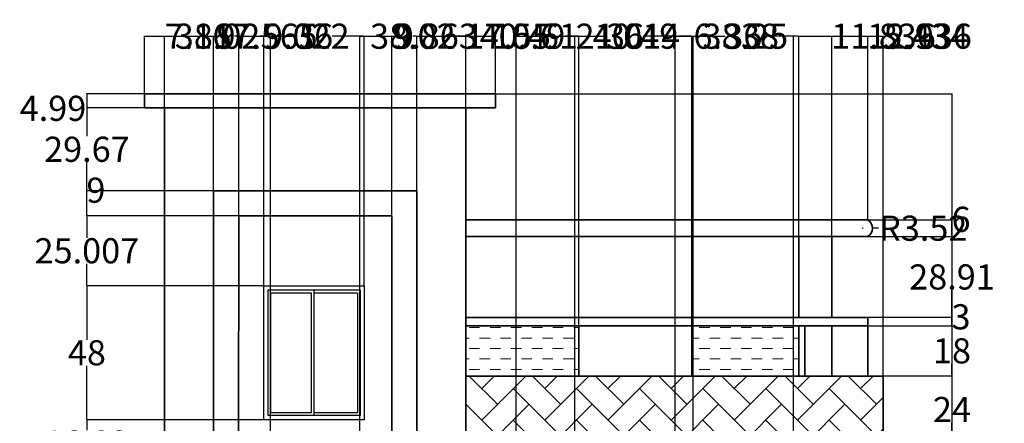
# Model space of a CAD drawing. Units: inches. Extents: x -30 to 323, y -174 to 256.
# Tile 4 of 4: x -30 to 323, y 112 to 256. Entities that reach past the tile are written whole.
import ezdxf

# ---------------------------------------------------------------- set-up
doc = ezdxf.new("R2010")
doc.units = ezdxf.units.IN
doc.header["$MEASUREMENT"] = 0
for name, color, linetype, lineweight in [('A-ANNO-DIMS', 2, 'Continuous', 18), ('A-ELEV', 7, 'Continuous', 35), ('A-ELEV-PATT', 8, 'Continuous', 13), ('A-GLAZ', 3, 'Continuous', 25)]:
    doc.layers.add(name, color=color, linetype=linetype, lineweight=lineweight)
doc.styles.get("Standard").update_dxf_attribs({"font": 'arial.ttf'})
doc.dimstyles.get("Standard").update_dxf_attribs({"dimtxt": 9, "dimasz": 0.18, "dimexe": 0.18, "dimexo": 0.0625, "dimgap": 0.09, "dimtad": 0, "dimtih": 1, "dimtoh": 1, "dimdec": 0, "dimzin": 0, "dimdsep": 46, "dimlunit": 3, "dimtxsty": 'Standard', "dimcen": 0.09, "dimadec": 0, "dimazin": 0, "dimtfac": 1, "dimtdec": 0, "dimtofl": 0, "dimtmove": 0, "dimatfit": 3, "dimfxl": 1, "dimtolj": 1, "dimtzin": 0, "dimarcsym": 0})

# ---------------------------------------------------------------- blocks, each defined once
blk = doc.blocks.new('*U2')
for p, q in [((1.5, 1.5), (1.5, 46.5)), ((1.5, 46.5), (18, 46.5)), ((18, 1.5), (18, 46.5)), ((18, 46.5), (34.5, 46.5)), ((34.5, 46.5), (34.5, 1.5)), ((18, 1.5), (1.5, 1.5)), ((34.5, 1.5), (18, 1.5))]:
    blk.add_line(p, q)
blk.add_lwpolyline([(0, 0), (0, 48), (36, 48), (36, 0)], close=True)
for points in [[(17, 45.5), (17, 2.5), (2.5, 2.5), (2.5, 45.5), (17, 45.5)], [(18, 45.5), (33.5, 45.5), (33.5, 2.5), (18, 2.5)]]:
    blk.add_lwpolyline(points)
blk = doc.blocks.new('*D10')
at = {"layer": 'A-ANNO-DIMS', "color": 0, "lineweight": -2, "transparency": 16777216}
for p, q in [((15.03, 229.9), (304.46, 229.9)), ((304.28, 229.72), (304.28, 50.56)), ((304.28, -137.97), (304.28, 41.18)), ((22.2, -138.15), (304.46, -138.15))]:
    blk.add_line(p, q, dxfattribs=at)
at = {"layer": 'A-ANNO-DIMS', "color": 0, "transparency": 16777216}
for points in [[(304.25, 229.72), (304.31, 229.72), (304.28, 229.9)], [(304.25, -137.97), (304.31, -137.97), (304.28, -138.15)]]:
    blk.add_solid(points, dxfattribs=at)
at = {"layer": 'Defpoints', "color": 0, "transparency": 16777216}
for p in [(14.97, 229.9), (22.14, -138.15), (304.28, -138.15)]:
    blk.add_point(p, dxfattribs=at)
at = {"layer": 'A-ANNO-DIMS', "color": 0, "transparency": 16777216, "insert": (304.28, 45.87), "char_height": 9, "attachment_point": 5}
blk.add_mtext('\\A1;368.05', dxfattribs=at)
blk = doc.blocks.new('*D11')
at = {"layer": 'A-ANNO-DIMS', "color": 0, "lineweight": -2, "transparency": 16777216}
for p, q in [((14.91, 229.9), (-5.86, 229.9)), ((-5.68, 229.72), (-5.68, 225.09)), ((22.07, 224.91), (-5.86, 224.91)), ((-5.68, 224.73), (-5.86, 224.73)), ((-5.68, 224.91), (-5.68, 224.73))]:
    blk.add_line(p, q, dxfattribs=at)
at = {"layer": 'A-ANNO-DIMS', "color": 0, "transparency": 16777216}
for points in [[(-5.71, 229.72), (-5.65, 229.72), (-5.68, 229.9)], [(-5.71, 225.09), (-5.65, 225.09), (-5.68, 224.91)]]:
    blk.add_solid(points, dxfattribs=at)
at = {"layer": 'Defpoints', "color": 0, "transparency": 16777216}
for p in [(14.97, 229.9), (-5.68, 224.91), (22.14, 224.91)]:
    blk.add_point(p, dxfattribs=at)
at = {"layer": 'A-ANNO-DIMS', "color": 0, "transparency": 16777216, "insert": (-17.83, 224.73), "char_height": 9, "attachment_point": 5}
blk.add_mtext('\\A1;4.99', dxfattribs=at)
blk = doc.blocks.new('*D12')
at = {"layer": 'A-ANNO-DIMS', "color": 0, "lineweight": -2, "transparency": 16777216}
for p, q in [((14.97, 224.97), (14.97, 250.73)), ((15.15, 250.55), (21.96, 250.55)), ((22.14, 224.97), (22.14, 250.73)), ((22.14, 250.55), (22.32, 250.55))]:
    blk.add_line(p, q, dxfattribs=at)
at = {"layer": 'A-ANNO-DIMS', "color": 0, "transparency": 16777216}
for points in [[(15.15, 250.58), (15.15, 250.52), (14.97, 250.55)], [(21.96, 250.58), (21.96, 250.52), (22.14, 250.55)]]:
    blk.add_solid(points, dxfattribs=at)
at = {"layer": 'Defpoints', "color": 0, "transparency": 16777216}
for p in [(22.14, 250.55), (14.97, 224.91), (22.14, 224.91)]:
    blk.add_point(p, dxfattribs=at)
at = {"layer": 'A-ANNO-DIMS', "color": 0, "transparency": 16777216, "insert": (37.55, 250.55), "char_height": 9, "attachment_point": 5}
blk.add_mtext('\\A1;7.167', dxfattribs=at)
blk = doc.blocks.new('*D13')
at = {"layer": 'A-ANNO-DIMS', "color": 0, "lineweight": -2, "transparency": 16777216}
for p, q in [((22.14, 224.97), (22.14, 250.73)), ((22.32, 250.55), (39.52, 250.55)), ((39.7, 195.3), (39.7, 250.73)), ((39.7, 250.55), (39.88, 250.55))]:
    blk.add_line(p, q, dxfattribs=at)
at = {"layer": 'A-ANNO-DIMS', "color": 0, "transparency": 16777216}
for points in [[(22.32, 250.58), (22.32, 250.52), (22.14, 250.55)], [(39.52, 250.58), (39.52, 250.52), (39.7, 250.55)]]:
    blk.add_solid(points, dxfattribs=at)
at = {"layer": 'Defpoints', "color": 0, "transparency": 16777216}
for p in [(39.7, 250.55), (22.14, 224.91), (39.7, 195.23)]:
    blk.add_point(p, dxfattribs=at)
at = {"layer": 'A-ANNO-DIMS', "color": 0, "transparency": 16777216, "insert": (58.26, 250.55), "char_height": 9, "attachment_point": 5}
blk.add_mtext('\\A1;17.565', dxfattribs=at)
blk = doc.blocks.new('*D14')
at = {"layer": 'A-ANNO-DIMS', "color": 0, "lineweight": -2, "transparency": 16777216}
for p, q in [((39.7, 195.3), (39.7, 250.73)), ((39.88, 250.55), (41.15, 250.55)), ((48.52, 250.55), (47.25, 250.55)), ((48.7, 186.3), (48.7, 250.73))]:
    blk.add_line(p, q, dxfattribs=at)
at = {"layer": 'A-ANNO-DIMS', "color": 0, "transparency": 16777216}
for points in [[(39.88, 250.58), (39.88, 250.52), (39.7, 250.55)], [(48.52, 250.58), (48.52, 250.52), (48.7, 250.55)]]:
    blk.add_solid(points, dxfattribs=at)
at = {"layer": 'Defpoints', "color": 0, "transparency": 16777216}
for p in [(48.7, 250.55), (39.7, 195.23), (48.7, 186.23)]:
    blk.add_point(p, dxfattribs=at)
at = {"layer": 'A-ANNO-DIMS', "color": 0, "transparency": 16777216, "insert": (44.2, 250.55), "char_height": 9, "attachment_point": 5}
blk.add_mtext('\\A1;9', dxfattribs=at)
blk = doc.blocks.new('*D15')
at = {"layer": 'A-ANNO-DIMS', "color": 0, "lineweight": -2, "transparency": 16777216}
for p, q in [((48.7, 186.3), (48.7, 250.73)), ((48.88, 250.55), (57.54, 250.55)), ((57.72, 161.29), (57.72, 250.73)), ((57.72, 250.55), (57.9, 250.55))]:
    blk.add_line(p, q, dxfattribs=at)
at = {"layer": 'A-ANNO-DIMS', "color": 0, "transparency": 16777216}
for points in [[(48.88, 250.58), (48.88, 250.52), (48.7, 250.55)], [(57.54, 250.58), (57.54, 250.52), (57.72, 250.55)]]:
    blk.add_solid(points, dxfattribs=at)
at = {"layer": 'Defpoints', "color": 0, "transparency": 16777216}
for p in [(57.72, 250.55), (48.7, 186.23), (57.72, 161.23)]:
    blk.add_point(p, dxfattribs=at)
at = {"layer": 'A-ANNO-DIMS', "color": 0, "transparency": 16777216, "insert": (73.13, 250.55), "char_height": 9, "attachment_point": 5}
blk.add_mtext('\\A1;9.022', dxfattribs=at)
blk = doc.blocks.new('*D16')
at = {"layer": 'A-ANNO-DIMS', "color": 0, "lineweight": -2, "transparency": 16777216}
for p, q in [((57.72, 161.29), (57.72, 250.73)), ((57.9, 250.55), (69.19, 250.55)), ((93.54, 250.55), (82.25, 250.55)), ((93.72, 161.29), (93.72, 250.73))]:
    blk.add_line(p, q, dxfattribs=at)
at = {"layer": 'A-ANNO-DIMS', "color": 0, "transparency": 16777216}
for points in [[(57.9, 250.58), (57.9, 250.52), (57.72, 250.55)], [(93.54, 250.58), (93.54, 250.52), (93.72, 250.55)]]:
    blk.add_solid(points, dxfattribs=at)
at = {"layer": 'Defpoints', "color": 0, "transparency": 16777216}
for p in [(93.72, 250.55), (57.72, 161.23), (93.72, 161.23)]:
    blk.add_point(p, dxfattribs=at)
at = {"layer": 'A-ANNO-DIMS', "color": 0, "transparency": 16777216, "insert": (75.72, 250.55), "char_height": 9, "attachment_point": 5}
blk.add_mtext('\\A1;36', dxfattribs=at)
blk = doc.blocks.new('*D17')
at = {"layer": 'A-ANNO-DIMS', "color": 0, "lineweight": -2, "transparency": 16777216}
for p, q in [((93.72, 161.29), (93.72, 250.73)), ((93.9, 250.55), (103.41, 250.55)), ((103.59, 186.3), (103.59, 250.73)), ((103.59, 250.55), (103.77, 250.55))]:
    blk.add_line(p, q, dxfattribs=at)
at = {"layer": 'A-ANNO-DIMS', "color": 0, "transparency": 16777216}
for points in [[(93.9, 250.58), (93.9, 250.52), (93.72, 250.55)], [(103.41, 250.58), (103.41, 250.52), (103.59, 250.55)]]:
    blk.add_solid(points, dxfattribs=at)
at = {"layer": 'Defpoints', "color": 0, "transparency": 16777216}
for p in [(103.59, 250.55), (103.59, 186.23), (93.72, 161.23)]:
    blk.add_point(p, dxfattribs=at)
at = {"layer": 'A-ANNO-DIMS', "color": 0, "transparency": 16777216, "insert": (119.04, 250.55), "char_height": 9, "attachment_point": 5}
blk.add_mtext('\\A1;9.863', dxfattribs=at)
blk = doc.blocks.new('*D18')
at = {"layer": 'A-ANNO-DIMS', "color": 0, "lineweight": -2, "transparency": 16777216}
for p, q in [((103.59, 186.3), (103.59, 250.73)), ((103.77, 250.55), (105.04, 250.55)), ((112.41, 250.55), (111.13, 250.55)), ((112.59, 195.3), (112.59, 250.73))]:
    blk.add_line(p, q, dxfattribs=at)
at = {"layer": 'A-ANNO-DIMS', "color": 0, "transparency": 16777216}
for points in [[(103.77, 250.58), (103.77, 250.52), (103.59, 250.55)], [(112.41, 250.58), (112.41, 250.52), (112.59, 250.55)]]:
    blk.add_solid(points, dxfattribs=at)
at = {"layer": 'Defpoints', "color": 0, "transparency": 16777216}
for p in [(112.59, 250.55), (112.59, 195.23), (103.59, 186.23)]:
    blk.add_point(p, dxfattribs=at)
at = {"layer": 'A-ANNO-DIMS', "color": 0, "transparency": 16777216, "insert": (108.09, 250.55), "char_height": 9, "attachment_point": 5}
blk.add_mtext('\\A1;9', dxfattribs=at)
blk = doc.blocks.new('*D19')
at = {"layer": 'A-ANNO-DIMS', "color": 0, "lineweight": -2, "transparency": 16777216}
for p, q in [((112.59, 195.3), (112.59, 250.73)), ((112.77, 250.55), (129.96, 250.55)), ((130.14, 224.97), (130.14, 250.73)), ((130.14, 250.55), (130.32, 250.55))]:
    blk.add_line(p, q, dxfattribs=at)
at = {"layer": 'A-ANNO-DIMS', "color": 0, "transparency": 16777216}
for points in [[(112.77, 250.58), (112.77, 250.52), (112.59, 250.55)], [(129.96, 250.58), (129.96, 250.52), (130.14, 250.55)]]:
    blk.add_solid(points, dxfattribs=at)
at = {"layer": 'Defpoints', "color": 0, "transparency": 16777216}
for p in [(130.14, 250.55), (130.14, 224.91), (112.59, 195.23)]:
    blk.add_point(p, dxfattribs=at)
at = {"layer": 'A-ANNO-DIMS', "color": 0, "transparency": 16777216, "insert": (145.2, 250.55), "char_height": 9, "attachment_point": 5}
blk.add_mtext('\\A1;17.55', dxfattribs=at)
blk = doc.blocks.new('*D20')
at = {"layer": 'A-ANNO-DIMS', "color": 0, "lineweight": -2, "transparency": 16777216}
for p, q in [((130.14, 224.97), (130.14, 250.73)), ((130.32, 250.55), (140.57, 250.55)), ((140.75, 224.97), (140.75, 250.73)), ((140.75, 250.55), (140.93, 250.55))]:
    blk.add_line(p, q, dxfattribs=at)
at = {"layer": 'A-ANNO-DIMS', "color": 0, "transparency": 16777216}
for points in [[(130.32, 250.58), (130.32, 250.52), (130.14, 250.55)], [(140.57, 250.58), (140.57, 250.52), (140.75, 250.55)]]:
    blk.add_solid(points, dxfattribs=at)
at = {"layer": 'Defpoints', "color": 0, "transparency": 16777216}
for p in [(140.75, 250.55), (130.14, 224.91), (140.75, 224.91)]:
    blk.add_point(p, dxfattribs=at)
at = {"layer": 'A-ANNO-DIMS', "color": 0, "transparency": 16777216, "insert": (154.91, 250.55), "char_height": 9, "attachment_point": 5}
blk.add_mtext('\\A1;10.61', dxfattribs=at)
blk = doc.blocks.new('*D21')
at = {"layer": 'A-ANNO-DIMS', "color": 0, "lineweight": -2, "transparency": 16777216}
for p, q in [((22.14, -111.03), (22.14, 250.73)), ((22.32, 250.55), (25.92, 250.55)), ((59.97, 250.55), (56.37, 250.55)), ((60.15, -60.62), (60.15, 250.73))]:
    blk.add_line(p, q, dxfattribs=at)
at = {"layer": 'A-ANNO-DIMS', "color": 0, "transparency": 16777216}
for points in [[(22.32, 250.58), (22.32, 250.52), (22.14, 250.55)], [(59.97, 250.58), (59.97, 250.52), (60.15, 250.55)]]:
    blk.add_solid(points, dxfattribs=at)
at = {"layer": 'Defpoints', "color": 0, "transparency": 16777216}
for p in [(60.15, 250.55), (60.15, -60.68), (22.14, -111.09)]:
    blk.add_point(p, dxfattribs=at)
at = {"layer": 'A-ANNO-DIMS', "color": 0, "transparency": 16777216, "insert": (41.14, 250.55), "char_height": 9, "attachment_point": 5}
blk.add_mtext('\\A1;38.02', dxfattribs=at)
blk = doc.blocks.new('*D22')
at = {"layer": 'A-ANNO-DIMS', "color": 0, "lineweight": -2, "transparency": 16777216}
for p, q in [((92.12, -60.62), (92.12, 250.73)), ((92.3, 250.55), (95.9, 250.55)), ((129.96, 250.55), (126.35, 250.55)), ((130.14, -111.03), (130.14, 250.73))]:
    blk.add_line(p, q, dxfattribs=at)
at = {"layer": 'A-ANNO-DIMS', "color": 0, "transparency": 16777216}
for points in [[(92.3, 250.58), (92.3, 250.52), (92.12, 250.55)], [(129.96, 250.58), (129.96, 250.52), (130.14, 250.55)]]:
    blk.add_solid(points, dxfattribs=at)
at = {"layer": 'Defpoints', "color": 0, "transparency": 16777216}
for p in [(130.14, 250.55), (92.12, -60.68), (130.14, -111.09)]:
    blk.add_point(p, dxfattribs=at)
at = {"layer": 'A-ANNO-DIMS', "color": 0, "transparency": 16777216, "insert": (111.13, 250.55), "char_height": 9, "attachment_point": 5}
blk.add_mtext('\\A1;38.02', dxfattribs=at)
blk = doc.blocks.new('*D33')
at = {"layer": 'A-ANNO-DIMS', "color": 0, "lineweight": -2, "transparency": 16777216}
for p, q in [((57.66, 113.23), (-5.86, 113.23)), ((-5.68, 113.05), (-5.68, 109.5)), ((-5.68, 96.59), (-5.68, 100.13)), ((48.63, 96.41), (-5.86, 96.41))]:
    blk.add_line(p, q, dxfattribs=at)
at = {"layer": 'A-ANNO-DIMS', "color": 0, "transparency": 16777216}
for points in [[(-5.71, 113.05), (-5.65, 113.05), (-5.68, 113.23)], [(-5.71, 96.59), (-5.65, 96.59), (-5.68, 96.41)]]:
    blk.add_solid(points, dxfattribs=at)
at = {"layer": 'Defpoints', "color": 0, "transparency": 16777216}
for p in [(-5.68, 113.23), (57.72, 113.23), (48.7, 96.41)]:
    blk.add_point(p, dxfattribs=at)
at = {"layer": 'A-ANNO-DIMS', "color": 0, "transparency": 16777216, "insert": (-5.68, 104.82), "char_height": 9, "attachment_point": 5}
blk.add_mtext('\\A1;16.82', dxfattribs=at)
blk = doc.blocks.new('*D34')
at = {"layer": 'A-ANNO-DIMS', "color": 0, "lineweight": -2, "transparency": 16777216}
for p, q in [((57.66, 161.23), (-5.86, 161.23)), ((-5.68, 161.05), (-5.68, 141.91)), ((-5.68, 113.41), (-5.68, 132.54)), ((57.66, 113.23), (-5.86, 113.23))]:
    blk.add_line(p, q, dxfattribs=at)
at = {"layer": 'A-ANNO-DIMS', "color": 0, "transparency": 16777216}
for points in [[(-5.71, 161.05), (-5.65, 161.05), (-5.68, 161.23)], [(-5.71, 113.41), (-5.65, 113.41), (-5.68, 113.23)]]:
    blk.add_solid(points, dxfattribs=at)
at = {"layer": 'Defpoints', "color": 0, "transparency": 16777216}
for p in [(-5.68, 161.23), (57.72, 161.23), (57.72, 113.23)]:
    blk.add_point(p, dxfattribs=at)
at = {"layer": 'A-ANNO-DIMS', "color": 0, "transparency": 16777216, "insert": (-5.68, 137.23), "char_height": 9, "attachment_point": 5}
blk.add_mtext('\\A1;48', dxfattribs=at)
blk = doc.blocks.new('*D35')
at = {"layer": 'A-ANNO-DIMS', "color": 0, "lineweight": -2, "transparency": 16777216}
for p, q in [((48.64, 186.23), (-5.86, 186.23)), ((-5.68, 186.05), (-5.68, 178.42)), ((-5.68, 161.41), (-5.68, 169.05)), ((57.66, 161.23), (-5.86, 161.23))]:
    blk.add_line(p, q, dxfattribs=at)
at = {"layer": 'A-ANNO-DIMS', "color": 0, "transparency": 16777216}
for points in [[(-5.71, 186.05), (-5.65, 186.05), (-5.68, 186.23)], [(-5.71, 161.41), (-5.65, 161.41), (-5.68, 161.23)]]:
    blk.add_solid(points, dxfattribs=at)
at = {"layer": 'Defpoints', "color": 0, "transparency": 16777216}
for p in [(-5.68, 186.23), (48.7, 186.23), (57.72, 161.23)]:
    blk.add_point(p, dxfattribs=at)
at = {"layer": 'A-ANNO-DIMS', "color": 0, "transparency": 16777216, "insert": (-5.68, 173.73), "char_height": 9, "attachment_point": 5}
blk.add_mtext('\\A1;25.007', dxfattribs=at)
blk = doc.blocks.new('*D36')
at = {"layer": 'A-ANNO-DIMS', "color": 0, "lineweight": -2, "transparency": 16777216}
for p, q in [((39.64, 195.23), (-5.86, 195.23)), ((-5.68, 195.23), (-5.68, 195.41)), ((-5.68, 195.41), (-5.5, 195.41)), ((-5.68, 186.41), (-5.68, 195.05)), ((48.64, 186.23), (-5.86, 186.23))]:
    blk.add_line(p, q, dxfattribs=at)
at = {"layer": 'A-ANNO-DIMS', "color": 0, "transparency": 16777216}
for points in [[(-5.71, 195.05), (-5.65, 195.05), (-5.68, 195.23)], [(-5.71, 186.41), (-5.65, 186.41), (-5.68, 186.23)]]:
    blk.add_solid(points, dxfattribs=at)
at = {"layer": 'Defpoints', "color": 0, "transparency": 16777216}
for p in [(-5.68, 195.23), (39.7, 195.23), (48.7, 186.23)]:
    blk.add_point(p, dxfattribs=at)
at = {"layer": 'A-ANNO-DIMS', "color": 0, "transparency": 16777216, "insert": (-2.45, 195.41), "char_height": 9, "attachment_point": 5}
blk.add_mtext('\\A1;9', dxfattribs=at)
blk = doc.blocks.new('*D37')
at = {"layer": 'A-ANNO-DIMS', "color": 0, "lineweight": -2, "transparency": 16777216}
for p, q in [((22.07, 224.91), (-5.86, 224.91)), ((-5.68, 224.73), (-5.68, 214.76)), ((-5.68, 195.41), (-5.68, 205.38)), ((39.64, 195.23), (-5.86, 195.23))]:
    blk.add_line(p, q, dxfattribs=at)
at = {"layer": 'A-ANNO-DIMS', "color": 0, "transparency": 16777216}
for points in [[(-5.71, 224.73), (-5.65, 224.73), (-5.68, 224.91)], [(-5.71, 195.41), (-5.65, 195.41), (-5.68, 195.23)]]:
    blk.add_solid(points, dxfattribs=at)
at = {"layer": 'Defpoints', "color": 0, "transparency": 16777216}
for p in [(-5.68, 224.91), (22.14, 224.91), (39.7, 195.23)]:
    blk.add_point(p, dxfattribs=at)
at = {"layer": 'A-ANNO-DIMS', "color": 0, "transparency": 16777216, "insert": (-5.68, 210.07), "char_height": 9, "attachment_point": 5}
blk.add_mtext('\\A1;29.67', dxfattribs=at)
blk = doc.blocks.new('*D38')
at = {"layer": 'A-ANNO-DIMS', "color": 0, "lineweight": -2, "transparency": 16777216}
for p, q in [((130.14, 184.88), (130.14, 250.73)), ((130.32, 250.55), (134.92, 250.55)), ((170.45, 250.55), (165.85, 250.55)), ((170.63, 146.97), (170.63, 250.73))]:
    blk.add_line(p, q, dxfattribs=at)
at = {"layer": 'A-ANNO-DIMS', "color": 0, "transparency": 16777216}
for points in [[(130.32, 250.58), (130.32, 250.52), (130.14, 250.55)], [(170.45, 250.58), (170.45, 250.52), (170.63, 250.55)]]:
    blk.add_solid(points, dxfattribs=at)
at = {"layer": 'Defpoints', "color": 0, "transparency": 16777216}
for p in [(170.63, 250.55), (130.14, 184.82), (170.63, 146.91)]:
    blk.add_point(p, dxfattribs=at)
at = {"layer": 'A-ANNO-DIMS', "color": 0, "transparency": 16777216, "insert": (150.38, 250.55), "char_height": 9, "attachment_point": 5}
blk.add_mtext('\\A1;40.49', dxfattribs=at)
blk = doc.blocks.new('*D39')
at = {"layer": 'A-ANNO-DIMS', "color": 0, "lineweight": -2, "transparency": 16777216}
for p, q in [((170.63, 146.97), (170.63, 250.73)), ((170.81, 250.55), (175.4, 250.55)), ((210.93, 250.55), (206.34, 250.55)), ((211.11, 146.97), (211.11, 250.73))]:
    blk.add_line(p, q, dxfattribs=at)
at = {"layer": 'A-ANNO-DIMS', "color": 0, "transparency": 16777216}
for points in [[(170.81, 250.58), (170.81, 250.52), (170.63, 250.55)], [(210.93, 250.58), (210.93, 250.52), (211.11, 250.55)]]:
    blk.add_solid(points, dxfattribs=at)
at = {"layer": 'Defpoints', "color": 0, "transparency": 16777216}
for p in [(211.11, 250.55), (170.63, 146.91), (211.11, 146.91)]:
    blk.add_point(p, dxfattribs=at)
at = {"layer": 'A-ANNO-DIMS', "color": 0, "transparency": 16777216, "insert": (190.87, 250.55), "char_height": 9, "attachment_point": 5}
blk.add_mtext('\\A1;40.49', dxfattribs=at)
blk = doc.blocks.new('*D40')
at = {"layer": 'A-ANNO-DIMS', "color": 0, "lineweight": -2, "transparency": 16777216}
for p, q in [((211.11, 146.97), (211.11, 250.73)), ((211.29, 250.55), (214.93, 250.55)), ((249.18, 250.55), (245.54, 250.55)), ((249.36, 178.88), (249.36, 250.73))]:
    blk.add_line(p, q, dxfattribs=at)
at = {"layer": 'A-ANNO-DIMS', "color": 0, "transparency": 16777216}
for points in [[(211.29, 250.58), (211.29, 250.52), (211.11, 250.55)], [(249.18, 250.58), (249.18, 250.52), (249.36, 250.55)]]:
    blk.add_solid(points, dxfattribs=at)
at = {"layer": 'Defpoints', "color": 0, "transparency": 16777216}
for p in [(249.36, 250.55), (249.36, 178.82), (211.11, 146.91)]:
    blk.add_point(p, dxfattribs=at)
at = {"layer": 'A-ANNO-DIMS', "color": 0, "transparency": 16777216, "insert": (230.24, 250.55), "char_height": 9, "attachment_point": 5}
blk.add_mtext('\\A1;38.25', dxfattribs=at)
blk = doc.blocks.new('*D41')
at = {"layer": 'A-ANNO-DIMS', "color": 0, "lineweight": -2, "transparency": 16777216}
for p, q in [((249.36, 178.88), (249.36, 250.73)), ((249.54, 250.55), (261.02, 250.55)), ((261.2, 178.88), (261.2, 250.73)), ((261.2, 250.55), (261.38, 250.55))]:
    blk.add_line(p, q, dxfattribs=at)
at = {"layer": 'A-ANNO-DIMS', "color": 0, "transparency": 16777216}
for points in [[(249.54, 250.58), (249.54, 250.52), (249.36, 250.55)], [(261.02, 250.58), (261.02, 250.52), (261.2, 250.55)]]:
    blk.add_solid(points, dxfattribs=at)
at = {"layer": 'Defpoints', "color": 0, "transparency": 16777216}
for p in [(261.2, 250.55), (249.36, 178.82), (261.2, 178.82)]:
    blk.add_point(p, dxfattribs=at)
at = {"layer": 'A-ANNO-DIMS', "color": 0, "transparency": 16777216, "insert": (279.72, 250.55), "char_height": 9, "attachment_point": 5}
blk.add_mtext('\\A1;11.836', dxfattribs=at)
blk = doc.blocks.new('*D42')
at = {"layer": 'A-ANNO-DIMS', "color": 0, "lineweight": -2, "transparency": 16777216}
for p, q in [((261.2, 178.88), (261.2, 250.73)), ((261.38, 250.55), (273.96, 250.55)), ((274.14, 184.88), (274.14, 250.73)), ((274.14, 250.55), (274.32, 250.55))]:
    blk.add_line(p, q, dxfattribs=at)
at = {"layer": 'A-ANNO-DIMS', "color": 0, "transparency": 16777216}
for points in [[(261.38, 250.58), (261.38, 250.52), (261.2, 250.55)], [(273.96, 250.58), (273.96, 250.52), (274.14, 250.55)]]:
    blk.add_solid(points, dxfattribs=at)
at = {"layer": 'Defpoints', "color": 0, "transparency": 16777216}
for p in [(274.14, 250.55), (274.14, 184.82), (261.2, 178.82)]:
    blk.add_point(p, dxfattribs=at)
at = {"layer": 'A-ANNO-DIMS', "color": 0, "transparency": 16777216, "insert": (292.66, 250.55), "char_height": 9, "attachment_point": 5}
blk.add_mtext('\\A1;12.936', dxfattribs=at)
blk = doc.blocks.new('*D43')
at = {"layer": 'A-ANNO-DIMS', "color": 0, "lineweight": -2, "transparency": 16777216}
for p, q in [((274.14, 184.88), (274.14, 250.73)), ((274.32, 250.55), (279.39, 250.55)), ((279.57, 128.97), (279.57, 250.73)), ((279.57, 250.55), (279.75, 250.55))]:
    blk.add_line(p, q, dxfattribs=at)
at = {"layer": 'A-ANNO-DIMS', "color": 0, "transparency": 16777216}
for points in [[(274.32, 250.58), (274.32, 250.52), (274.14, 250.55)], [(279.39, 250.58), (279.39, 250.52), (279.57, 250.55)]]:
    blk.add_solid(points, dxfattribs=at)
at = {"layer": 'Defpoints', "color": 0, "transparency": 16777216}
for p in [(279.57, 250.55), (274.14, 184.82), (279.57, 128.91)]:
    blk.add_point(p, dxfattribs=at)
at = {"layer": 'A-ANNO-DIMS', "color": 0, "transparency": 16777216, "insert": (295.01, 250.55), "char_height": 9, "attachment_point": 5}
blk.add_mtext('\\A1;5.434', dxfattribs=at)
blk = doc.blocks.new('*D52')
at = {"layer": 'A-ANNO-DIMS', "color": 0, "lineweight": -2, "transparency": 16777216}
for p, q in [((148.14, -47.95), (148.14, 250.73)), ((148.32, 250.55), (168.97, 250.55)), ((169.15, -13.98), (169.15, 250.73)), ((169.15, 250.55), (169.33, 250.55))]:
    blk.add_line(p, q, dxfattribs=at)
at = {"layer": 'A-ANNO-DIMS', "color": 0, "transparency": 16777216}
for points in [[(148.32, 250.58), (148.32, 250.52), (148.14, 250.55)], [(168.97, 250.58), (168.97, 250.52), (169.15, 250.55)]]:
    blk.add_solid(points, dxfattribs=at)
at = {"layer": 'Defpoints', "color": 0, "transparency": 16777216}
for p in [(169.15, 250.55), (169.15, -14.04), (148.14, -48.01)]:
    blk.add_point(p, dxfattribs=at)
at = {"layer": 'A-ANNO-DIMS', "color": 0, "transparency": 16777216, "insert": (188.16, 250.55), "char_height": 9, "attachment_point": 5}
blk.add_mtext('\\A1;21.014', dxfattribs=at)
blk = doc.blocks.new('*D53')
at = {"layer": 'A-ANNO-DIMS', "color": 0, "lineweight": -2, "transparency": 16777216}
for p, q in [((169.15, -13.98), (169.15, 250.73)), ((169.33, 250.55), (180.62, 250.55)), ((204.97, 250.55), (193.68, 250.55)), ((205.15, -13.98), (205.15, 250.73))]:
    blk.add_line(p, q, dxfattribs=at)
at = {"layer": 'A-ANNO-DIMS', "color": 0, "transparency": 16777216}
for points in [[(169.33, 250.58), (169.33, 250.52), (169.15, 250.55)], [(204.97, 250.58), (204.97, 250.52), (205.15, 250.55)]]:
    blk.add_solid(points, dxfattribs=at)
at = {"layer": 'Defpoints', "color": 0, "transparency": 16777216}
for p in [(205.15, 250.55), (169.15, -14.04), (205.15, -14.04)]:
    blk.add_point(p, dxfattribs=at)
at = {"layer": 'A-ANNO-DIMS', "color": 0, "transparency": 16777216, "insert": (187.15, 250.55), "char_height": 9, "attachment_point": 5}
blk.add_mtext('\\A1;36', dxfattribs=at)
blk = doc.blocks.new('*D54')
at = {"layer": 'A-ANNO-DIMS', "color": 0, "lineweight": -2, "transparency": 16777216}
for p, q in [((205.15, -13.98), (205.15, 250.73)), ((205.33, 250.55), (211.31, 250.55)), ((211.49, -13.74), (211.49, 250.73)), ((211.49, 250.55), (211.67, 250.55))]:
    blk.add_line(p, q, dxfattribs=at)
at = {"layer": 'A-ANNO-DIMS', "color": 0, "transparency": 16777216}
for points in [[(205.33, 250.58), (205.33, 250.52), (205.15, 250.55)], [(211.31, 250.58), (211.31, 250.52), (211.49, 250.55)]]:
    blk.add_solid(points, dxfattribs=at)
at = {"layer": 'Defpoints', "color": 0, "transparency": 16777216}
for p in [(211.49, 250.55), (205.15, -14.04), (211.49, -13.8)]:
    blk.add_point(p, dxfattribs=at)
at = {"layer": 'A-ANNO-DIMS', "color": 0, "transparency": 16777216, "insert": (226.98, 250.55), "char_height": 9, "attachment_point": 5}
blk.add_mtext('\\A1;6.338', dxfattribs=at)
blk = doc.blocks.new('*D55')
at = {"layer": 'A-ANNO-DIMS', "color": 0, "lineweight": -2, "transparency": 16777216}
for p, q in [((211.49, -13.74), (211.49, 250.73)), ((211.67, 250.55), (222.96, 250.55)), ((247.31, 250.55), (236.02, 250.55)), ((247.49, -13.74), (247.49, 250.73))]:
    blk.add_line(p, q, dxfattribs=at)
at = {"layer": 'A-ANNO-DIMS', "color": 0, "transparency": 16777216}
for points in [[(211.67, 250.58), (211.67, 250.52), (211.49, 250.55)], [(247.31, 250.58), (247.31, 250.52), (247.49, 250.55)]]:
    blk.add_solid(points, dxfattribs=at)
at = {"layer": 'Defpoints', "color": 0, "transparency": 16777216}
for p in [(247.49, 250.55), (211.49, -13.8), (247.49, -13.8)]:
    blk.add_point(p, dxfattribs=at)
at = {"layer": 'A-ANNO-DIMS', "color": 0, "transparency": 16777216, "insert": (229.49, 250.55), "char_height": 9, "attachment_point": 5}
blk.add_mtext('\\A1;36', dxfattribs=at)
blk = doc.blocks.new('*D69')
at = {"layer": 'A-ANNO-DIMS', "color": 0, "lineweight": -2, "transparency": 16777216}
for p, q in [((279.63, 128.91), (304.46, 128.91)), ((304.28, 128.73), (304.28, 121.51)), ((304.28, 105.09), (304.28, 112.3)), ((279.63, 104.91), (304.46, 104.91))]:
    blk.add_line(p, q, dxfattribs=at)
at = {"layer": 'A-ANNO-DIMS', "color": 0, "transparency": 16777216}
for points in [[(304.25, 128.73), (304.31, 128.73), (304.28, 128.91)], [(304.25, 105.09), (304.31, 105.09), (304.28, 104.91)]]:
    blk.add_solid(points, dxfattribs=at)
at = {"layer": 'Defpoints', "color": 0, "transparency": 16777216}
for p in [(279.57, 128.91), (304.28, 128.91), (279.57, 104.91)]:
    blk.add_point(p, dxfattribs=at)
at = {"layer": 'A-ANNO-DIMS', "color": 0, "transparency": 16777216, "insert": (304.28, 116.91), "char_height": 9, "attachment_point": 5}
blk.add_mtext('\\A1;24', dxfattribs=at)
blk = doc.blocks.new('*D70')
at = {"layer": 'A-ANNO-DIMS', "color": 0, "lineweight": -2, "transparency": 16777216}
for p, q in [((274.2, 146.91), (304.46, 146.91)), ((304.28, 146.73), (304.28, 142.59)), ((304.28, 129.09), (304.28, 133.22)), ((274.2, 128.91), (304.46, 128.91))]:
    blk.add_line(p, q, dxfattribs=at)
at = {"layer": 'A-ANNO-DIMS', "color": 0, "transparency": 16777216}
for points in [[(304.25, 146.73), (304.31, 146.73), (304.28, 146.91)], [(304.25, 129.09), (304.31, 129.09), (304.28, 128.91)]]:
    blk.add_solid(points, dxfattribs=at)
at = {"layer": 'Defpoints', "color": 0, "transparency": 16777216}
for p in [(274.14, 146.91), (304.28, 146.91), (274.14, 128.91)]:
    blk.add_point(p, dxfattribs=at)
at = {"layer": 'A-ANNO-DIMS', "color": 0, "transparency": 16777216, "insert": (304.28, 137.91), "char_height": 9, "attachment_point": 5}
blk.add_mtext('\\A1;18', dxfattribs=at)
blk = doc.blocks.new('*D71')
at = {"layer": 'A-ANNO-DIMS', "color": 0, "lineweight": -2, "transparency": 16777216}
for p, q in [((274.2, 149.91), (304.46, 149.91)), ((304.28, 149.91), (304.28, 150.09)), ((304.28, 150.09), (304.46, 150.09)), ((304.28, 147.09), (304.28, 149.73)), ((274.2, 146.91), (304.46, 146.91))]:
    blk.add_line(p, q, dxfattribs=at)
at = {"layer": 'A-ANNO-DIMS', "color": 0, "transparency": 16777216}
for points in [[(304.25, 149.73), (304.31, 149.73), (304.28, 149.91)], [(304.25, 147.09), (304.31, 147.09), (304.28, 146.91)]]:
    blk.add_solid(points, dxfattribs=at)
at = {"layer": 'Defpoints', "color": 0, "transparency": 16777216}
for p in [(274.14, 149.91), (304.28, 149.91), (274.14, 146.91)]:
    blk.add_point(p, dxfattribs=at)
at = {"layer": 'A-ANNO-DIMS', "color": 0, "transparency": 16777216, "insert": (307.5, 150.09), "char_height": 9, "attachment_point": 5}
blk.add_mtext('\\A1;3', dxfattribs=at)
blk = doc.blocks.new('*D72')
at = {"layer": 'A-ANNO-DIMS', "color": 0, "lineweight": -2, "transparency": 16777216}
for p, q in [((261.26, 178.82), (304.46, 178.82)), ((304.28, 178.64), (304.28, 169.05)), ((304.28, 150.09), (304.28, 159.68)), ((261.26, 149.91), (304.46, 149.91))]:
    blk.add_line(p, q, dxfattribs=at)
at = {"layer": 'A-ANNO-DIMS', "color": 0, "transparency": 16777216}
for points in [[(304.25, 178.64), (304.31, 178.64), (304.28, 178.82)], [(304.25, 150.09), (304.31, 150.09), (304.28, 149.91)]]:
    blk.add_solid(points, dxfattribs=at)
at = {"layer": 'Defpoints', "color": 0, "transparency": 16777216}
for p in [(261.2, 178.82), (304.28, 178.82), (261.2, 149.91)]:
    blk.add_point(p, dxfattribs=at)
at = {"layer": 'A-ANNO-DIMS', "color": 0, "transparency": 16777216, "insert": (304.28, 164.36), "char_height": 9, "attachment_point": 5}
blk.add_mtext('\\A1;28.91', dxfattribs=at)
blk = doc.blocks.new('*D73')
at = {"layer": 'A-ANNO-DIMS', "color": 0, "lineweight": -2, "transparency": 16777216}
for p, q in [((274.2, 184.82), (304.46, 184.82)), ((304.28, 184.82), (304.28, 185)), ((304.28, 185), (304.46, 185)), ((304.28, 179), (304.28, 184.64)), ((261.26, 178.82), (304.46, 178.82))]:
    blk.add_line(p, q, dxfattribs=at)
at = {"layer": 'A-ANNO-DIMS', "color": 0, "transparency": 16777216}
for points in [[(304.25, 184.64), (304.31, 184.64), (304.28, 184.82)], [(304.25, 179), (304.31, 179), (304.28, 178.82)]]:
    blk.add_solid(points, dxfattribs=at)
at = {"layer": 'Defpoints', "color": 0, "transparency": 16777216}
for p in [(274.14, 184.82), (304.28, 184.82), (261.2, 178.82)]:
    blk.add_point(p, dxfattribs=at)
at = {"layer": 'A-ANNO-DIMS', "color": 0, "transparency": 16777216, "insert": (307.52, 185), "char_height": 9, "attachment_point": 5}
blk.add_mtext('\\A1;6', dxfattribs=at)
blk = doc.blocks.new('*D78')
at = {"layer": 'A-ANNO-DIMS', "color": 0, "lineweight": -2, "transparency": 16777216}
for p, q in [((272.21, 181.82), (272.39, 181.82)), ((272.3, 181.73), (272.3, 181.91)), ((277.93, 181.82), (276, 181.82))]:
    blk.add_line(p, q, dxfattribs=at)
at = {"layer": 'A-ANNO-DIMS', "color": 0, "transparency": 16777216}
blk.add_solid([(276, 181.85), (276, 181.79), (275.82, 181.82)], dxfattribs=at)
at = {"layer": 'Defpoints', "color": 0, "transparency": 16777216}
for p in [(272.3, 181.82), (275.82, 181.82)]:
    blk.add_point(p, dxfattribs=at)
at = {"layer": 'A-ANNO-DIMS', "color": 0, "transparency": 16777216, "insert": (293.97, 181.82), "char_height": 9, "attachment_point": 5}
blk.add_mtext('\\A1;R3.52', dxfattribs=at)

msp = doc.modelspace()

# ---------------------------------------------------------------- hatches: boundary and pattern name
at = {"layer": 'A-ELEV-PATT'}
h = msp.add_hatch(dxfattribs=at)
h.set_pattern_fill('DASH', color=256, scale=30)
h.paths.add_polyline_path([(170.6252, 146.9059), (130.136, 146.9059), (130.136, 128.9059), (170.6252, 128.9059)])
h.paths.add_polyline_path([(249.3636, 146.9059), (211.1144, 146.9059), (211.1144, 128.9059), (249.3636, 128.9059)])
h = msp.add_hatch(dxfattribs=at)
h.set_pattern_fill('AR-HBONE', color=256, scale=2)
h.paths.add_polyline_path([(279.5695, 128.9059), (274.136, 128.9059), (130.136, 128.9059), (130.136, 8.9059), (274.136, 8.9059), (283.6325, 8.9059), (283.6325, 20.9059), (274.136, 20.9059), (142.136, 20.9059), (142.136, 104.9059), (274.136, 104.9059), (279.5695, 104.9059)])

# ---------------------------------------------------------------- linework, layer by layer
at = {"layer": 'A-ELEV'}
for p, q in [((39.6938, -26.6189), (39.7012, 195.2341)), ((39.7012, 195.2341), (112.5855, 195.2341)), ((112.5855, 195.2341), (112.5782, -26.6189)), ((48.6941, -17.6189), (48.7009, 186.2341)), ((48.7009, 186.2341), (103.5852, 186.2341)), ((103.5852, 186.2341), (103.5785, -17.6189)), ((274.136, 146.9059), (130.136, 146.9059)), ((170.6252, 146.9059), (170.6252, 128.9059)), ((211.1144, 146.9059), (211.1144, 128.9059)), ((251.6036, 146.9059), (251.6036, 128.9059)), ((274.136, 128.9059), (130.136, 128.9059))]:
    msp.add_line(p, q, dxfattribs=at)
msp.add_lwpolyline([(14.9689, 224.9059), (140.747, 224.9059), (140.747, 229.8957), (14.9689, 229.8957)], close=True, dxfattribs=at)
for points in [[(130.136, 149.9059), (274.136, 149.9059), (274.136, 128.9059), (279.5695, 128.9059), (279.5695, 104.9059), (274.136, 104.9059), (274.136, 20.9059), (283.6325, 20.9059), (283.6325, 8.9059), (274.136, 8.9059), (274.136, -111.0941), (22.136, -111.0941), (22.136, 224.9059), (130.136, 224.9059), (130.136, -111.0941)], [(261.1996, 149.9059), (261.1996, 178.8161), (249.3636, 178.8161), (249.3636, 149.9059)], [(249.3636, 146.9059), (249.3636, 128.9059), (261.1996, 128.9059), (261.1996, 146.9059)]]:
    msp.add_lwpolyline(points, dxfattribs=at)
msp.add_lwpolyline([(130.136, 178.8161), (274.136, 178.8161, 0.56035554), (274.136, 184.8161), (130.136, 184.8161)], format="xyb", dxfattribs=at)

# ---------------------------------------------------------------- block references
at = {"layer": 'A-GLAZ'}
msp.add_blockref('*U2', (57.7226, 113.2271), dxfattribs=at)

# ---------------------------------------------------------------- dimensions: what is measured, and where the dimension line sits
at = {"layer": 'A-ANNO-DIMS'}
for base, p1, p2, override, picture, middle in [((22.136, 250.5457), (14.9689, 224.9059), (22.136, 224.9059), {"dimdec": 3, "dimlfac": 1, "dimrnd": 0, "dimzin": 0, "dimdsep": 46, "dimlunit": 2}, '*D12', (37.5543, 250.5457)), ((39.7012, 250.5457), (22.136, 224.9059), (39.7012, 195.2341), {"dimdec": 3, "dimlfac": 1, "dimrnd": 0, "dimzin": 0, "dimdsep": 46, "dimlunit": 2}, '*D13', (58.2628, 250.5457)), ((60.1531, 250.5457), (22.136, -111.0941), (60.1531, -60.6838), {"dimdec": 2, "dimlfac": 1, "dimrnd": 0, "dimzin": 0, "dimdsep": 46, "dimlunit": 2}, '*D21', (41.1445, 250.5457)), ((48.7009, 250.5457), (39.7012, 195.2341), (48.7009, 186.2341), {"dimdec": 0, "dimlfac": 1, "dimrnd": 0, "dimzin": 0, "dimdsep": 46, "dimlunit": 2}, '*D14', (44.201, 250.5457)), ((57.7226, 250.5457), (48.7009, 186.2341), (57.7226, 161.2271), {"dimdec": 3, "dimlfac": 1, "dimrnd": 0, "dimzin": 0, "dimdsep": 46, "dimlunit": 2}, '*D15', (73.1317, 250.5457)), ((93.7226, 250.5457), (57.7226, 161.2271), (93.7226, 161.2271), {"dimdec": 0, "dimlfac": 1, "dimrnd": 0, "dimzin": 0, "dimdsep": 46, "dimlunit": 2}, '*D16', (75.7226, 250.5457)), ((130.136, 250.5457), (92.1189, -60.6838), (130.136, -111.0941), {"dimdec": 2, "dimlfac": 1, "dimrnd": 0, "dimzin": 0, "dimdsep": 46, "dimlunit": 2}, '*D22', (111.1274, 250.5457)), ((103.5852, 250.5457), (93.7226, 161.2271), (103.5852, 186.2341), {"dimdec": 3, "dimlfac": 1, "dimrnd": 0, "dimzin": 0, "dimdsep": 46, "dimlunit": 2}, '*D17', (119.0404, 250.5457)), ((112.5855, 250.5457), (103.5852, 186.2341), (112.5855, 195.2341), {"dimdec": 0, "dimlfac": 1, "dimrnd": 0, "dimzin": 0, "dimdsep": 46, "dimlunit": 2}, '*D18', (108.0854, 250.5457)), ((130.136, 250.5457), (112.5855, 195.2341), (130.136, 224.9059), {"dimdec": 2, "dimlfac": 1, "dimrnd": 0, "dimzin": 0, "dimdsep": 46, "dimlunit": 2}, '*D19', (145.2013, 250.5457)), ((140.747, 250.5457), (130.136, 224.9059), (140.747, 224.9059), {"dimdec": 2, "dimlfac": 1, "dimrnd": 0, "dimzin": 0, "dimdsep": 46, "dimlunit": 2}, '*D20', (154.9099, 250.5457)), ((170.6252, 250.5457), (130.136, 184.8161), (170.6252, 146.9059), {"dimdec": 2, "dimlfac": 1, "dimrnd": 0, "dimzin": 0, "dimdsep": 46, "dimlunit": 2}, '*D38', (150.3806, 250.5457)), ((169.1503, 250.5457), (148.136, -48.0084), (169.1503, -14.04), {"dimdec": 3, "dimlfac": 1, "dimrnd": 0, "dimzin": 0, "dimdsep": 46, "dimlunit": 2}, '*D52', (188.1601, 250.5457)), ((205.1503, 250.5457), (169.1503, -14.04), (205.1503, -14.04), {"dimdec": 0, "dimlfac": 1, "dimrnd": 0, "dimzin": 0, "dimdsep": 46, "dimlunit": 2}, '*D53', (187.1503, 250.5457)), ((211.1144, 250.5457), (170.6252, 146.9059), (211.1144, 146.9059), {"dimdec": 2, "dimlfac": 1, "dimrnd": 0, "dimzin": 0, "dimdsep": 46, "dimlunit": 2}, '*D39', (190.8698, 250.5457)), ((211.4887, 250.5457), (205.1503, -14.04), (211.4887, -13.801), {"dimdec": 3, "dimlfac": 1, "dimrnd": 0, "dimzin": 0, "dimdsep": 46, "dimlunit": 2}, '*D54', (226.9777, 250.5457)), ((249.3636, 250.5457), (211.1144, 146.9059), (249.3636, 178.8161), {"dimdec": 2, "dimlfac": 1, "dimrnd": 0, "dimzin": 0, "dimdsep": 46, "dimlunit": 2}, '*D40', (230.239, 250.5457)), ((247.4887, 250.5457), (211.4887, -13.801), (247.4887, -13.801), {"dimdec": 0, "dimlfac": 1, "dimrnd": 0, "dimzin": 0, "dimdsep": 46, "dimlunit": 2}, '*D55', (229.4887, 250.5457)), ((261.1996, 250.5457), (249.3636, 178.8161), (261.1996, 178.8161), {"dimdec": 3, "dimlfac": 1, "dimrnd": 0, "dimzin": 0, "dimdsep": 46, "dimlunit": 2}, '*D41', (279.7243, 250.5457)), ((274.136, 250.5457), (261.1996, 178.8161), (274.136, 184.8161), {"dimdec": 3, "dimlfac": 1, "dimrnd": 0, "dimzin": 0, "dimdsep": 46, "dimlunit": 2}, '*D42', (292.6608, 250.5457)), ((279.569477, 250.545678), (274.135976, 184.816132), (279.569477, 128.905916), {"dimdec": 3, "dimlfac": 1, "dimrnd": 0, "dimzin": 0, "dimdsep": 46, "dimlunit": 2}, '*D43', (295.006257, 250.545678))]:
    dim = msp.add_linear_dim(base=base, p1=p1, p2=p2, dimstyle='Standard', override=override, dxfattribs=at)
    dim.commit()
    dim.dimension.update_dxf_attribs({"geometry": picture, "text_midpoint": middle})
for base, p1, p2, override, picture, middle in [((-5.6811, 224.9059), (14.9689, 229.8957), (22.136, 224.9059), {"dimdec": 2, "dimlfac": 1, "dimrnd": 0, "dimzin": 0, "dimdsep": 46, "dimlunit": 2}, '*D11', (-17.8303, 224.7259)), ((304.2825, -138.1526), (14.9689, 229.8957), (22.136, -138.1526), {"dimdec": 2, "dimlfac": 1, "dimrnd": 0, "dimzin": 0, "dimdsep": 46, "dimlunit": 2}, '*D10', (304.2825, 45.8715)), ((-5.6811, 224.9059), (39.7012, 195.2341), (22.136, 224.9059), {"dimdec": 2, "dimlfac": 1, "dimrnd": 0, "dimzin": 0, "dimdsep": 46, "dimlunit": 2}, '*D37', (-5.6811, 210.07)), ((-5.6811, 195.2341), (48.7009, 186.2341), (39.7012, 195.2341), {"dimdec": 0, "dimlfac": 1, "dimrnd": 0, "dimzin": 0, "dimdsep": 46, "dimlunit": 2}, '*D36', (-2.452, 195.4141)), ((304.2825, 184.8161), (261.1996, 178.8161), (274.136, 184.8161), {"dimdec": 0, "dimlfac": 1, "dimrnd": 0, "dimzin": 0, "dimdsep": 46, "dimlunit": 2}, '*D73', (307.5239, 184.9961)), ((-5.6811, 186.2341), (57.7226, 161.2271), (48.7009, 186.2341), {"dimdec": 3, "dimlfac": 1, "dimrnd": 0, "dimzin": 0, "dimdsep": 46, "dimlunit": 2}, '*D35', (-5.6811, 173.7306)), ((304.2825, 178.8161), (261.1996, 149.9059), (261.1996, 178.8161), {"dimdec": 2, "dimlfac": 1, "dimrnd": 0, "dimzin": 0, "dimdsep": 46, "dimlunit": 2}, '*D72', (304.2825, 164.361)), ((-5.6811, 161.2271), (57.7226, 113.2271), (57.7226, 161.2271), {"dimdec": 0, "dimlfac": 1, "dimrnd": 0, "dimzin": 0, "dimdsep": 46, "dimlunit": 2}, '*D34', (-5.6811, 137.2271)), ((304.2825, 149.9059), (274.136, 146.9059), (274.136, 149.9059), {"dimdec": 0, "dimlfac": 1, "dimrnd": 0, "dimzin": 0, "dimdsep": 46, "dimlunit": 2}, '*D71', (307.4993, 150.0859)), ((304.2825, 146.9059), (274.136, 128.9059), (274.136, 146.9059), {"dimdec": 0, "dimlfac": 1, "dimrnd": 0, "dimzin": 0, "dimdsep": 46, "dimlunit": 2}, '*D70', (304.2825, 137.9059)), ((304.2825, 128.9059), (279.5695, 104.9059), (279.5695, 128.9059), {"dimdec": 0, "dimlfac": 1, "dimrnd": 0, "dimzin": 0, "dimdsep": 46, "dimlunit": 2}, '*D69', (304.2825, 116.9059)), ((-5.6811, 113.2271), (48.6966, 96.4058), (57.7226, 113.2271), {"dimdec": 2, "dimlfac": 1, "dimrnd": 0, "dimzin": 0, "dimdsep": 46, "dimlunit": 2}, '*D33', (-5.6811, 104.8165))]:
    dim = msp.add_linear_dim(base=base, p1=p1, p2=p2, angle=90, dimstyle='Standard', override=override, dxfattribs=at)
    dim.commit()
    dim.dimension.update_dxf_attribs({"geometry": picture, "text_midpoint": middle})
dim = msp.add_radius_dim(center=(272.2996, 181.8161), mpoint=(275.817, 181.816), dimstyle='Standard', override={"dimdec": 2, "dimlfac": 1, "dimrnd": 0, "dimzin": 0, "dimdsep": 46, "dimlunit": 2}, dxfattribs=at)
dim.commit()
dim.dimension.update_dxf_attribs({"geometry": '*D78', "text_midpoint": (277.9275, 181.8159), "dimtype": 164})

doc.saveas('drawing.dxf')
